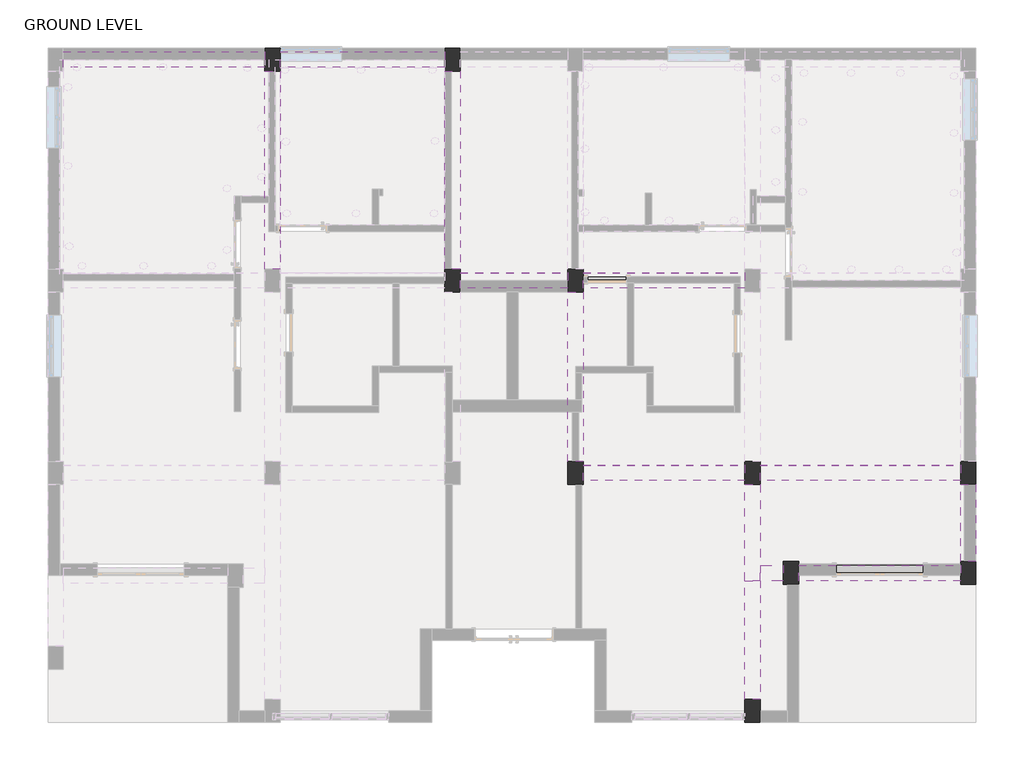
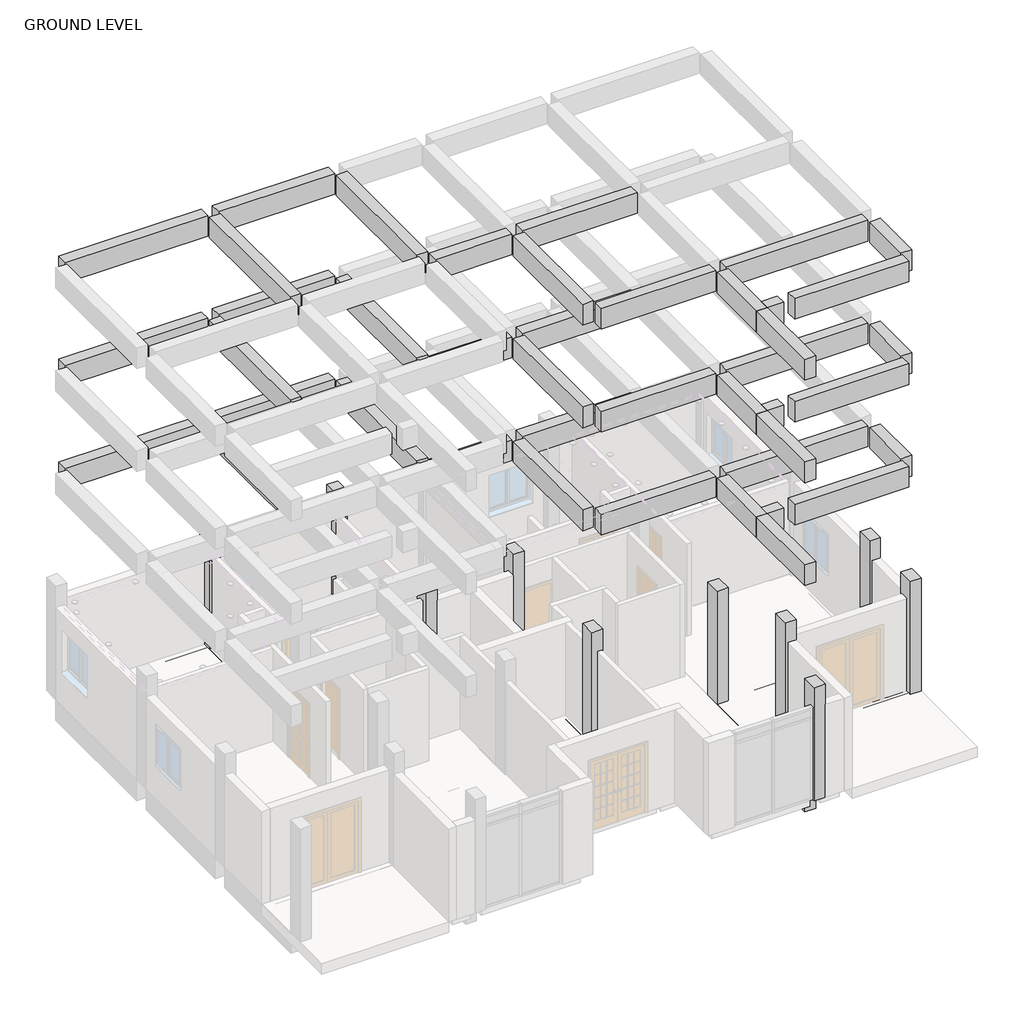
# One storey, part 4 of 5: 57 beams, 10 columns.
"""IFC4 building model written with IfcOpenShell, lengths in millimetres."""

from ifc_helpers import new_model, si_unit, frame, origin, origin_with_axes, place, context, project, spatial, polyline, outline, extrude, faceted_brep, element, save

model = new_model("IFC4")

# Units and contexts
model_context = context("Model", 3, world=origin())
ifc_project = project(units=[si_unit("LENGTHUNIT", "METRE", prefix="MILLI")], contexts=[model_context])

# Site, building, storey
site = spatial("IfcSite", under=ifc_project)
building = spatial("IfcBuilding", under=site)
storey = spatial("IfcBuildingStorey", under=building, Name="GROUND LEVEL", Elevation=0.0)

# Beams
placement = place(None, origin())
element("IfcBeam", 1, ObjectType="Concrete-Rectangular Beam : 12 x 24", at=placement, inside=storey, context=model_context, shape_type="SweptSolid", body=[
    extrude(outline(polyline([(-8839.9786397, -1604.6061634), (-8839.9786397, -1299.8061634), (-4852.9175798, -1299.8061634), (-4852.9175798, -1604.6061634), (-8839.9786397, -1604.6061634)])), frame((0.0, 0.0, -609.6), z_axis=(0.0, 0.0, 1.0), x_axis=(1.0, 0.0, 0.0)), (0.0, 0.0, 1.0), 609.6),
])
element("IfcBeam", 2, ObjectType="Concrete-Rectangular Beam : 12 x 24", at=placement, inside=storey, context=model_context, shape_type="SweptSolid", body=[
    extrude(outline(polyline([(-1296.9175798, -1299.8061634), (-1296.9175798, -1604.6061634), (-4548.1175798, -1604.6061634), (-4548.1175798, -1299.8061634), (-1296.9175798, -1299.8061634)])), frame((0.0, 0.0, -609.6), z_axis=(0.0, 0.0, 1.0), x_axis=(1.0, 0.0, 0.0)), (0.0, 0.0, 1.0), 609.6),
])
element("IfcBeam", 3, ObjectType="Concrete-Rectangular Beam : 12 x 24", at=placement, inside=storey, context=model_context, shape_type="SweptSolid", body=[
    extrude(outline(polyline([(9218.6824202, -11391.8620333), (8913.8824202, -11391.8620333), (8913.8824202, -9867.8620333), (9218.6824202, -9867.8620333), (9218.6824202, -11391.8620333)])), frame((0.0, 0.0, -609.6), z_axis=(0.0, 0.0, 1.0), x_axis=(1.0, 0.0, 0.0)), (0.0, 0.0, 1.0), 609.6),
])
element("IfcBeam", 4, ObjectType="Concrete-Rectangular Beam : 12 x 24", at=placement, inside=storey, context=model_context, shape_type="SweptSolid", body=[
    extrude(outline(polyline([(1446.2824202, -5981.6620333), (1446.2824202, -5676.8620333), (4646.6824202, -5676.8620333), (4646.6824202, -5981.6620333), (1446.2824202, -5981.6620333)])), frame((0.0, 0.0, -609.6), z_axis=(0.0, 0.0, 1.0), x_axis=(1.0, 0.0, 0.0)), (0.0, 0.0, 1.0), 609.6),
])
element("IfcBeam", 5, ObjectType="Concrete-Rectangular Beam : 12 x 24", at=placement, inside=storey, context=model_context, shape_type="SweptSolid", body=[
    extrude(outline(polyline([(-992.1175798, -5981.6620333), (-992.1175798, -5676.8620333), (1141.4824202, -5676.8620333), (1141.4824202, -5981.6620333), (-992.1175798, -5981.6620333)])), frame((0.0, 0.0, -609.6), z_axis=(0.0, 0.0, 1.0), x_axis=(1.0, 0.0, 0.0)), (0.0, 0.0, 1.0), 609.6),
])
element("IfcBeam", 6, ObjectType="Concrete-Rectangular Beam : 12 x 24", at=placement, inside=storey, context=model_context, shape_type="SweptSolid", body=[
    extrude(outline(polyline([(1141.4824202, -9486.8620333), (1141.4824202, -9791.6620333), (-992.1175798, -9791.6620333), (-992.1175798, -9486.8620333), (1141.4824202, -9486.8620333)])), frame((0.0, 0.0, -609.6), z_axis=(0.0, 0.0, 1.0), x_axis=(1.0, 0.0, 0.0)), (0.0, 0.0, 1.0), 609.6),
])
element("IfcBeam", 7, ObjectType="Concrete-Rectangular Beam : 12 x 24", at=placement, inside=storey, context=model_context, shape_type="SweptSolid", body=[
    extrude(outline(polyline([(1446.2824202, -9791.6620333), (1446.2824202, -9486.8620333), (4646.6824202, -9486.8620333), (4646.6824202, -9791.6620333), (1446.2824202, -9791.6620333)])), frame((0.0, 0.0, -609.6), z_axis=(0.0, 0.0, 1.0), x_axis=(1.0, 0.0, 0.0)), (0.0, 0.0, 1.0), 609.6),
])
element("IfcBeam", 8, ObjectType="Concrete-Rectangular Beam : 12 x 24", at=placement, inside=storey, context=model_context, shape_type="Brep", body=[
    faceted_brep([(4951.4824202, -9867.8620333, 0.0), (4646.6824202, -9867.8620333, 0.0), (4646.6824202, -11772.8620333, 0.0), (4951.4824202, -11772.8620333, 0.0), (4951.4824202, -11468.0620333, 0.0), (4646.6824202, -9867.8620333, -609.6), (4646.6824202, -11772.8620333, -609.6), (4951.4824202, -9867.8620333, -609.6), (4951.4824202, -11468.0620333, -609.6), (4951.4824202, -11772.8620333, -609.6)], [[[0, 1, 2, 3, 4]], [[1, 5, 6, 2]], [[5, 7, 8, 9, 6]], [[7, 0, 4, 3, 9, 8]], [[0, 7, 5, 1]], [[3, 2, 6, 9]]]),
])
element("IfcBeam", 9, ObjectType="Concrete-Rectangular Beam : 12 x 24", at=placement, inside=storey, context=model_context, shape_type="SweptSolid", body=[
    extrude(outline(polyline([(5408.6824202, -11468.0620333), (5408.6824202, -11772.8620333), (4951.4824202, -11772.8620333), (4951.4824202, -11468.0620333), (5408.6824202, -11468.0620333)])), frame((0.0, 0.0, -609.6), z_axis=(0.0, 0.0, 1.0), x_axis=(1.0, 0.0, 0.0)), (0.0, 0.0, 1.0), 609.6),
])
element("IfcBeam", 10, ObjectType="Concrete-Rectangular Beam : 12 x 24", at=placement, inside=storey, context=model_context, shape_type="SweptSolid", body=[
    extrude(outline(polyline([(8913.8824202, -11468.0620333), (8913.8824202, -11772.8620333), (5713.4824202, -11772.8620333), (5713.4824202, -11468.0620333), (8913.8824202, -11468.0620333)])), frame((0.0, 0.0, -609.6), z_axis=(0.0, 0.0, 1.0), x_axis=(1.0, 0.0, 0.0)), (0.0, 0.0, 1.0), 609.6),
])
element("IfcBeam", 11, ObjectType="Concrete-Rectangular Beam : 12 x 24", at=placement, inside=storey, context=model_context, shape_type="SweptSolid", body=[
    extrude(outline(polyline([(4951.4824202, -14119.6402089), (4646.6824202, -14119.6402089), (4646.6824202, -11772.8620333), (4951.4824202, -11772.8620333), (4951.4824202, -14119.6402089)])), frame((0.0, 0.0, -609.6), z_axis=(0.0, 0.0, 1.0), x_axis=(1.0, 0.0, 0.0)), (0.0, 0.0, 1.0), 609.6),
])
element("IfcBeam", 12, ObjectType="Concrete-Rectangular Beam : 12 x 24", at=placement, inside=storey, context=model_context, shape_type="SweptSolid", body=[
    extrude(outline(polyline([(-4548.1175798, -5600.6620333), (-4852.9175798, -5600.6620333), (-4852.9175798, -1680.8061634), (-4548.1175798, -1680.8061634), (-4548.1175798, -5600.6620333)])), frame((0.0, 0.0, -609.6), z_axis=(0.0, 0.0, 1.0), x_axis=(1.0, 0.0, 0.0)), (0.0, 0.0, 1.0), 609.6),
])
element("IfcBeam", 13, ObjectType="Concrete-Rectangular Beam : 12 x 24", at=placement, inside=storey, context=model_context, shape_type="SweptSolid", body=[
    extrude(outline(polyline([(-992.1175798, -5600.6620333), (-1296.9175798, -5600.6620333), (-1296.9175798, -1680.8061634), (-992.1175798, -1680.8061634), (-992.1175798, -5600.6620333)])), frame((0.0, 0.0, -609.6), z_axis=(0.0, 0.0, 1.0), x_axis=(1.0, 0.0, 0.0)), (0.0, 0.0, 1.0), 609.6),
])
element("IfcBeam", 14, ObjectType="Concrete-Rectangular Beam : 12 x 24", at=placement, inside=storey, context=model_context, shape_type="SweptSolid", body=[
    extrude(outline(polyline([(1141.4824202, -6057.8620333), (1446.2824202, -6057.8620333), (1446.2824202, -9410.6620333), (1141.4824202, -9410.6620333), (1141.4824202, -6057.8620333)])), frame((0.0, 0.0, -609.6), z_axis=(0.0, 0.0, 1.0), x_axis=(1.0, 0.0, 0.0)), (0.0, 0.0, 1.0), 609.6),
])
element("IfcBeam", 15, ObjectType="Concrete-Rectangular Beam : 12 x 24", at=placement, inside=storey, context=model_context, shape_type="SweptSolid", body=[
    extrude(outline(polyline([(4951.4824202, -9791.6620333), (4951.4824202, -9486.8620333), (8913.8824202, -9486.8620333), (8913.8824202, -9791.6620333), (4951.4824202, -9791.6620333)])), frame((0.0, 0.0, -609.6), z_axis=(0.0, 0.0, 1.0), x_axis=(1.0, 0.0, 0.0)), (0.0, 0.0, 1.0), 609.6),
])
element("IfcBeam", 16, ObjectType="Concrete-Rectangular Beam : 12 x 24", at=placement, inside=storey, context=model_context, shape_type="SweptSolid", body=[
    extrude(outline(polyline([(-8839.9786397, -1604.6061634), (-8839.9786397, -1299.8061634), (-4852.9175798, -1299.8061634), (-4852.9175798, -1604.6061634), (-8839.9786397, -1604.6061634)])), frame((0.0, 0.0, 6096.0), z_axis=(0.0, 0.0, 1.0), x_axis=(1.0, 0.0, 0.0)), (0.0, 0.0, 1.0), 609.6),
])
element("IfcBeam", 17, ObjectType="Concrete-Rectangular Beam : 12 x 24", at=placement, inside=storey, context=model_context, shape_type="SweptSolid", body=[
    extrude(outline(polyline([(-1296.9175798, -1299.8061634), (-1296.9175798, -1604.6061634), (-4548.1175798, -1604.6061634), (-4548.1175798, -1299.8061634), (-1296.9175798, -1299.8061634)])), frame((0.0, 0.0, 6096.0), z_axis=(0.0, 0.0, 1.0), x_axis=(1.0, 0.0, 0.0)), (0.0, 0.0, 1.0), 609.6),
])
element("IfcBeam", 18, ObjectType="Concrete-Rectangular Beam : 12 x 24", at=placement, inside=storey, context=model_context, shape_type="Brep", body=[
    faceted_brep([(8913.8824202, -11391.8620333, 6705.6), (9218.6824202, -11391.8620333, 6705.6), (9218.6824202, -9867.8620333, 6705.6), (8913.8824202, -9867.8620333, 6705.6), (8913.8824202, -11391.8620333, 6096.0), (8913.8824202, -11391.8620333, 6400.8), (8913.8824202, -9867.8620333, 6400.8), (8913.8824202, -9867.8620333, 6096.0), (9218.6824202, -11391.8620333, 6096.0), (9218.6824202, -9867.8620333, 6096.0), (9218.6824202, -11391.8620333, 6400.8), (9218.6824202, -9867.8620333, 6400.8)], [[[0, 1, 2, 3]], [[4, 5, 0, 3, 6, 7]], [[8, 4, 7, 9]], [[1, 10, 8, 9, 11, 2]], [[1, 0, 5, 4, 8, 10]], [[2, 11, 9, 7, 6, 3]]]),
])
element("IfcBeam", 19, ObjectType="Concrete-Rectangular Beam : 12 x 24", at=placement, inside=storey, context=model_context, shape_type="SweptSolid", body=[
    extrude(outline(polyline([(1446.2824202, -5981.6620333), (1446.2824202, -5676.8620333), (4646.6824202, -5676.8620333), (4646.6824202, -5981.6620333), (1446.2824202, -5981.6620333)])), frame((0.0, 0.0, 6096.0), z_axis=(0.0, 0.0, 1.0), x_axis=(1.0, 0.0, 0.0)), (0.0, 0.0, 1.0), 609.6),
])
element("IfcBeam", 20, ObjectType="Concrete-Rectangular Beam : 12 x 24", at=placement, inside=storey, context=model_context, shape_type="SweptSolid", body=[
    extrude(outline(polyline([(-992.1175798, -5981.6620333), (-992.1175798, -5676.8620333), (1141.4824202, -5676.8620333), (1141.4824202, -5981.6620333), (-992.1175798, -5981.6620333)])), frame((0.0, 0.0, 6096.0), z_axis=(0.0, 0.0, 1.0), x_axis=(1.0, 0.0, 0.0)), (0.0, 0.0, 1.0), 609.6),
])
element("IfcBeam", 21, ObjectType="Concrete-Rectangular Beam : 12 x 24", at=placement, inside=storey, context=model_context, shape_type="SweptSolid", body=[
    extrude(outline(polyline([(1446.2824202, -9791.6620333), (1446.2824202, -9486.8620333), (4646.6824202, -9486.8620333), (4646.6824202, -9791.6620333), (1446.2824202, -9791.6620333)])), frame((0.0, 0.0, 6096.0), z_axis=(0.0, 0.0, 1.0), x_axis=(1.0, 0.0, 0.0)), (0.0, 0.0, 1.0), 609.6),
])
element("IfcBeam", 22, ObjectType="Concrete-Rectangular Beam : 12 x 24", at=placement, inside=storey, context=model_context, shape_type="Brep", body=[
    faceted_brep([(4951.4824202, -9867.8620333, 6705.6), (4646.6824202, -9867.8620333, 6705.6), (4646.6824202, -11772.8620333, 6705.6), (4951.4824202, -11772.8620333, 6705.6), (4951.4824202, -11468.0620333, 6705.6), (4646.6824202, -9867.8620333, 6400.8), (4646.6824202, -9867.8620333, 6096.0), (4646.6824202, -11772.8620333, 6096.0), (4951.4824202, -9867.8620333, 6096.0), (4951.4824202, -11468.0620333, 6096.0), (4951.4824202, -11772.8620333, 6096.0), (4951.4824202, -9867.8620333, 6400.8)], [[[0, 1, 2, 3, 4]], [[1, 5, 6, 7, 2]], [[6, 8, 9, 10, 7]], [[8, 11, 0, 4, 3, 10, 9]], [[0, 11, 8, 6, 5, 1]], [[3, 2, 7, 10]]]),
])
element("IfcBeam", 23, ObjectType="Concrete-Rectangular Beam : 12 x 24", at=placement, inside=storey, context=model_context, shape_type="SweptSolid", body=[
    extrude(outline(polyline([(5408.6824202, -11468.0620333), (5408.6824202, -11772.8620333), (4951.4824202, -11772.8620333), (4951.4824202, -11468.0620333), (5408.6824202, -11468.0620333)])), frame((0.0, 0.0, 6096.0), z_axis=(0.0, 0.0, 1.0), x_axis=(1.0, 0.0, 0.0)), (0.0, 0.0, 1.0), 609.6),
])
element("IfcBeam", 24, ObjectType="Concrete-Rectangular Beam : 12 x 24", at=placement, inside=storey, context=model_context, shape_type="SweptSolid", body=[
    extrude(outline(polyline([(8913.8824202, -11468.0620333), (8913.8824202, -11772.8620333), (5713.4824202, -11772.8620333), (5713.4824202, -11468.0620333), (8913.8824202, -11468.0620333)])), frame((0.0, 0.0, 6096.0), z_axis=(0.0, 0.0, 1.0), x_axis=(1.0, 0.0, 0.0)), (0.0, 0.0, 1.0), 609.6),
])
element("IfcBeam", 25, ObjectType="Concrete-Rectangular Beam : 12 x 24", at=placement, inside=storey, context=model_context, shape_type="Brep", body=[
    faceted_brep([(4646.6824202, -14119.6402089, 6705.6), (4951.4824202, -14119.6402089, 6705.6), (4951.4824202, -11772.8620333, 6705.6), (4646.6824202, -11772.8620333, 6705.6), (4951.4824202, -14119.6402089, 6400.8), (4951.4824202, -14119.6402089, 6096.0), (4951.4824202, -11772.8620333, 6096.0), (4646.6824202, -14119.6402089, 6096.0), (4646.6824202, -11772.8620333, 6096.0), (4646.6824202, -14119.6402089, 6400.8)], [[[0, 1, 2, 3]], [[1, 4, 5, 6, 2]], [[5, 7, 8, 6]], [[7, 9, 0, 3, 8]], [[0, 9, 7, 5, 4, 1]], [[3, 2, 6, 8]]]),
])
element("IfcBeam", 26, ObjectType="Concrete-Rectangular Beam : 12 x 24", at=placement, inside=storey, context=model_context, shape_type="Brep", body=[
    faceted_brep([(-4852.9175798, -5600.6620333, 6705.6), (-4548.1175798, -5600.6620333, 6705.6), (-4548.1175798, -1680.8061634, 6705.6), (-4852.9175798, -1680.8061634, 6705.6), (-4852.9175798, -5600.6620333, 6096.0), (-4852.9175798, -5600.6620333, 6400.8), (-4852.9175798, -1680.8061634, 6400.8), (-4852.9175798, -1680.8061634, 6096.0), (-4548.1175798, -5600.6620333, 6096.0), (-4548.1175798, -1680.8061634, 6096.0), (-4548.1175798, -5600.6620333, 6400.8), (-4548.1175798, -1680.8061634, 6400.8)], [[[0, 1, 2, 3]], [[4, 5, 0, 3, 6, 7]], [[8, 4, 7, 9]], [[1, 10, 8, 9, 11, 2]], [[2, 11, 9, 7, 6, 3]], [[1, 0, 5, 4, 8, 10]]]),
])
element("IfcBeam", 27, ObjectType="Concrete-Rectangular Beam : 12 x 24", at=placement, inside=storey, context=model_context, shape_type="Brep", body=[
    faceted_brep([(-1296.9175798, -5600.6620333, 6705.6), (-992.1175798, -5600.6620333, 6705.6), (-992.1175798, -1680.8061634, 6705.6), (-1296.9175798, -1680.8061634, 6705.6), (-1296.9175798, -5600.6620333, 6096.0), (-1296.9175798, -5600.6620333, 6400.8), (-1296.9175798, -1680.8061634, 6400.8), (-1296.9175798, -1680.8061634, 6096.0), (-992.1175798, -5600.6620333, 6096.0), (-992.1175798, -1680.8061634, 6096.0), (-992.1175798, -5600.6620333, 6400.8), (-992.1175798, -1680.8061634, 6400.8)], [[[0, 1, 2, 3]], [[4, 5, 0, 3, 6, 7]], [[8, 4, 7, 9]], [[1, 10, 8, 9, 11, 2]], [[2, 11, 9, 7, 6, 3]], [[1, 0, 5, 4, 8, 10]]]),
])
element("IfcBeam", 28, ObjectType="Concrete-Rectangular Beam : 12 x 24", at=placement, inside=storey, context=model_context, shape_type="Brep", body=[
    faceted_brep([(1446.2824202, -6057.8620333, 6705.6), (1141.4824202, -6057.8620333, 6705.6), (1141.4824202, -9410.6620333, 6705.6), (1446.2824202, -9410.6620333, 6705.6), (1446.2824202, -6057.8620333, 6096.0), (1446.2824202, -6057.8620333, 6400.8), (1446.2824202, -9410.6620333, 6400.8), (1446.2824202, -9410.6620333, 6096.0), (1141.4824202, -6057.8620333, 6096.0), (1141.4824202, -9410.6620333, 6096.0), (1141.4824202, -6057.8620333, 6400.8), (1141.4824202, -9410.6620333, 6400.8)], [[[0, 1, 2, 3]], [[4, 5, 0, 3, 6, 7]], [[8, 4, 7, 9]], [[1, 10, 8, 9, 11, 2]], [[1, 0, 5, 4, 8, 10]], [[2, 11, 9, 7, 6, 3]]]),
])
element("IfcBeam", 29, ObjectType="Concrete-Rectangular Beam : 12 x 24", at=placement, inside=storey, context=model_context, shape_type="SweptSolid", body=[
    extrude(outline(polyline([(4951.4824202, -9791.6620333), (4951.4824202, -9486.8620333), (8913.8824202, -9486.8620333), (8913.8824202, -9791.6620333), (4951.4824202, -9791.6620333)])), frame((0.0, 0.0, 6096.0), z_axis=(0.0, 0.0, 1.0), x_axis=(1.0, 0.0, 0.0)), (0.0, 0.0, 1.0), 609.6),
])
element("IfcBeam", 30, ObjectType="Concrete-Rectangular Beam : 12 x 24", at=placement, inside=storey, context=model_context, shape_type="SweptSolid", body=[
    extrude(outline(polyline([(-8839.9786397, -1604.6061634), (-8839.9786397, -1299.8061634), (-4852.9175798, -1299.8061634), (-4852.9175798, -1604.6061634), (-8839.9786397, -1604.6061634)])), frame((0.0, 0.0, 9144.0), z_axis=(0.0, 0.0, 1.0), x_axis=(1.0, 0.0, 0.0)), (0.0, 0.0, 1.0), 609.6),
])
element("IfcBeam", 31, ObjectType="Concrete-Rectangular Beam : 12 x 24", at=placement, inside=storey, context=model_context, shape_type="SweptSolid", body=[
    extrude(outline(polyline([(-1296.9175798, -1299.8061634), (-1296.9175798, -1604.6061634), (-4548.1175798, -1604.6061634), (-4548.1175798, -1299.8061634), (-1296.9175798, -1299.8061634)])), frame((0.0, 0.0, 9144.0), z_axis=(0.0, 0.0, 1.0), x_axis=(1.0, 0.0, 0.0)), (0.0, 0.0, 1.0), 609.6),
])
element("IfcBeam", 32, ObjectType="Concrete-Rectangular Beam : 12 x 24", at=placement, inside=storey, context=model_context, shape_type="Brep", body=[
    faceted_brep([(8913.8824202, -11391.8620333, 9753.6), (9218.6824202, -11391.8620333, 9753.6), (9218.6824202, -9867.8620333, 9753.6), (8913.8824202, -9867.8620333, 9753.6), (8913.8824202, -11391.8620333, 9144.0), (8913.8824202, -11391.8620333, 9448.8), (8913.8824202, -9867.8620333, 9448.8), (8913.8824202, -9867.8620333, 9144.0), (9218.6824202, -11391.8620333, 9144.0), (9218.6824202, -9867.8620333, 9144.0), (9218.6824202, -11391.8620333, 9448.8), (9218.6824202, -9867.8620333, 9448.8)], [[[0, 1, 2, 3]], [[4, 5, 0, 3, 6, 7]], [[8, 4, 7, 9]], [[1, 10, 8, 9, 11, 2]], [[1, 0, 5, 4, 8, 10]], [[2, 11, 9, 7, 6, 3]]]),
])
element("IfcBeam", 33, ObjectType="Concrete-Rectangular Beam : 12 x 24", at=placement, inside=storey, context=model_context, shape_type="SweptSolid", body=[
    extrude(outline(polyline([(1446.2824202, -5981.6620333), (1446.2824202, -5676.8620333), (4646.6824202, -5676.8620333), (4646.6824202, -5981.6620333), (1446.2824202, -5981.6620333)])), frame((0.0, 0.0, 9144.0), z_axis=(0.0, 0.0, 1.0), x_axis=(1.0, 0.0, 0.0)), (0.0, 0.0, 1.0), 609.6),
])
element("IfcBeam", 34, ObjectType="Concrete-Rectangular Beam : 12 x 24", at=placement, inside=storey, context=model_context, shape_type="SweptSolid", body=[
    extrude(outline(polyline([(-992.1175798, -5981.6620333), (-992.1175798, -5676.8620333), (1141.4824202, -5676.8620333), (1141.4824202, -5981.6620333), (-992.1175798, -5981.6620333)])), frame((0.0, 0.0, 9144.0), z_axis=(0.0, 0.0, 1.0), x_axis=(1.0, 0.0, 0.0)), (0.0, 0.0, 1.0), 609.6),
])
element("IfcBeam", 35, ObjectType="Concrete-Rectangular Beam : 12 x 24", at=placement, inside=storey, context=model_context, shape_type="SweptSolid", body=[
    extrude(outline(polyline([(1446.2824202, -9791.6620333), (1446.2824202, -9486.8620333), (4646.6824202, -9486.8620333), (4646.6824202, -9791.6620333), (1446.2824202, -9791.6620333)])), frame((0.0, 0.0, 9144.0), z_axis=(0.0, 0.0, 1.0), x_axis=(1.0, 0.0, 0.0)), (0.0, 0.0, 1.0), 609.6),
])
element("IfcBeam", 36, ObjectType="Concrete-Rectangular Beam : 12 x 24", at=placement, inside=storey, context=model_context, shape_type="Brep", body=[
    faceted_brep([(4951.4824202, -9867.8620333, 9753.6), (4646.6824202, -9867.8620333, 9753.6), (4646.6824202, -11772.8620333, 9753.6), (4951.4824202, -11772.8620333, 9753.6), (4951.4824202, -11468.0620333, 9753.6), (4646.6824202, -9867.8620333, 9448.8), (4646.6824202, -9867.8620333, 9144.0), (4646.6824202, -11772.8620333, 9144.0), (4951.4824202, -9867.8620333, 9144.0), (4951.4824202, -11468.0620333, 9144.0), (4951.4824202, -11772.8620333, 9144.0), (4951.4824202, -9867.8620333, 9448.8)], [[[0, 1, 2, 3, 4]], [[1, 5, 6, 7, 2]], [[6, 8, 9, 10, 7]], [[8, 11, 0, 4, 3, 10, 9]], [[0, 11, 8, 6, 5, 1]], [[3, 2, 7, 10]]]),
])
element("IfcBeam", 37, ObjectType="Concrete-Rectangular Beam : 12 x 24", at=placement, inside=storey, context=model_context, shape_type="SweptSolid", body=[
    extrude(outline(polyline([(5408.6824202, -11468.0620333), (5408.6824202, -11772.8620333), (4951.4824202, -11772.8620333), (4951.4824202, -11468.0620333), (5408.6824202, -11468.0620333)])), frame((0.0, 0.0, 9144.0), z_axis=(0.0, 0.0, 1.0), x_axis=(1.0, 0.0, 0.0)), (0.0, 0.0, 1.0), 609.6),
])
element("IfcBeam", 38, ObjectType="Concrete-Rectangular Beam : 12 x 24", at=placement, inside=storey, context=model_context, shape_type="SweptSolid", body=[
    extrude(outline(polyline([(8913.8824202, -11468.0620333), (8913.8824202, -11772.8620333), (5713.4824202, -11772.8620333), (5713.4824202, -11468.0620333), (8913.8824202, -11468.0620333)])), frame((0.0, 0.0, 9144.0), z_axis=(0.0, 0.0, 1.0), x_axis=(1.0, 0.0, 0.0)), (0.0, 0.0, 1.0), 609.6),
])
element("IfcBeam", 39, ObjectType="Concrete-Rectangular Beam : 12 x 24", at=placement, inside=storey, context=model_context, shape_type="Brep", body=[
    faceted_brep([(4646.6824202, -14119.6402089, 9753.6), (4951.4824202, -14119.6402089, 9753.6), (4951.4824202, -11772.8620333, 9753.6), (4646.6824202, -11772.8620333, 9753.6), (4951.4824202, -14119.6402089, 9448.8), (4951.4824202, -14119.6402089, 9144.0), (4951.4824202, -11772.8620333, 9144.0), (4646.6824202, -14119.6402089, 9144.0), (4646.6824202, -11772.8620333, 9144.0), (4646.6824202, -14119.6402089, 9448.8)], [[[0, 1, 2, 3]], [[1, 4, 5, 6, 2]], [[5, 7, 8, 6]], [[7, 9, 0, 3, 8]], [[0, 9, 7, 5, 4, 1]], [[3, 2, 6, 8]]]),
])
element("IfcBeam", 40, ObjectType="Concrete-Rectangular Beam : 12 x 24", at=placement, inside=storey, context=model_context, shape_type="Brep", body=[
    faceted_brep([(-4852.9175798, -5600.6620333, 9753.6), (-4548.1175798, -5600.6620333, 9753.6), (-4548.1175798, -1680.8061634, 9753.6), (-4852.9175798, -1680.8061634, 9753.6), (-4852.9175798, -5600.6620333, 9144.0), (-4852.9175798, -5600.6620333, 9448.8), (-4852.9175798, -1680.8061634, 9448.8), (-4852.9175798, -1680.8061634, 9144.0), (-4548.1175798, -5600.6620333, 9144.0), (-4548.1175798, -1680.8061634, 9144.0), (-4548.1175798, -5600.6620333, 9448.8), (-4548.1175798, -1680.8061634, 9448.8)], [[[0, 1, 2, 3]], [[4, 5, 0, 3, 6, 7]], [[8, 4, 7, 9]], [[1, 10, 8, 9, 11, 2]], [[2, 11, 9, 7, 6, 3]], [[1, 0, 5, 4, 8, 10]]]),
])
element("IfcBeam", 41, ObjectType="Concrete-Rectangular Beam : 12 x 24", at=placement, inside=storey, context=model_context, shape_type="Brep", body=[
    faceted_brep([(-1296.9175798, -5600.6620333, 9753.6), (-992.1175798, -5600.6620333, 9753.6), (-992.1175798, -1680.8061634, 9753.6), (-1296.9175798, -1680.8061634, 9753.6), (-1296.9175798, -5600.6620333, 9144.0), (-1296.9175798, -5600.6620333, 9448.8), (-1296.9175798, -1680.8061634, 9448.8), (-1296.9175798, -1680.8061634, 9144.0), (-992.1175798, -5600.6620333, 9144.0), (-992.1175798, -1680.8061634, 9144.0), (-992.1175798, -5600.6620333, 9448.8), (-992.1175798, -1680.8061634, 9448.8)], [[[0, 1, 2, 3]], [[4, 5, 0, 3, 6, 7]], [[8, 4, 7, 9]], [[1, 10, 8, 9, 11, 2]], [[2, 11, 9, 7, 6, 3]], [[1, 0, 5, 4, 8, 10]]]),
])
element("IfcBeam", 42, ObjectType="Concrete-Rectangular Beam : 12 x 24", at=placement, inside=storey, context=model_context, shape_type="Brep", body=[
    faceted_brep([(1446.2824202, -6057.8620333, 9753.6), (1141.4824202, -6057.8620333, 9753.6), (1141.4824202, -9410.6620333, 9753.6), (1446.2824202, -9410.6620333, 9753.6), (1446.2824202, -6057.8620333, 9144.0), (1446.2824202, -6057.8620333, 9448.8), (1446.2824202, -9410.6620333, 9448.8), (1446.2824202, -9410.6620333, 9144.0), (1141.4824202, -6057.8620333, 9144.0), (1141.4824202, -9410.6620333, 9144.0), (1141.4824202, -6057.8620333, 9448.8), (1141.4824202, -9410.6620333, 9448.8)], [[[0, 1, 2, 3]], [[4, 5, 0, 3, 6, 7]], [[8, 4, 7, 9]], [[1, 10, 8, 9, 11, 2]], [[1, 0, 5, 4, 8, 10]], [[2, 11, 9, 7, 6, 3]]]),
])
element("IfcBeam", 43, ObjectType="Concrete-Rectangular Beam : 12 x 24", at=placement, inside=storey, context=model_context, shape_type="SweptSolid", body=[
    extrude(outline(polyline([(4951.4824202, -9791.6620333), (4951.4824202, -9486.8620333), (8913.8824202, -9486.8620333), (8913.8824202, -9791.6620333), (4951.4824202, -9791.6620333)])), frame((0.0, 0.0, 9144.0), z_axis=(0.0, 0.0, 1.0), x_axis=(1.0, 0.0, 0.0)), (0.0, 0.0, 1.0), 609.6),
])
element("IfcBeam", 44, ObjectType="Concrete-Rectangular Beam : 12 x 24", at=placement, inside=storey, context=model_context, shape_type="SweptSolid", body=[
    extrude(outline(polyline([(-8839.9786397, -1604.6061634), (-8839.9786397, -1299.8061634), (-4852.9175798, -1299.8061634), (-4852.9175798, -1604.6061634), (-8839.9786397, -1604.6061634)])), frame((0.0, 0.0, 12192.0), z_axis=(0.0, 0.0, 1.0), x_axis=(1.0, 0.0, 0.0)), (0.0, 0.0, 1.0), 609.6),
])
element("IfcBeam", 45, ObjectType="Concrete-Rectangular Beam : 12 x 24", at=placement, inside=storey, context=model_context, shape_type="SweptSolid", body=[
    extrude(outline(polyline([(-1296.9175798, -1299.8061634), (-1296.9175798, -1604.6061634), (-4548.1175798, -1604.6061634), (-4548.1175798, -1299.8061634), (-1296.9175798, -1299.8061634)])), frame((0.0, 0.0, 12192.0), z_axis=(0.0, 0.0, 1.0), x_axis=(1.0, 0.0, 0.0)), (0.0, 0.0, 1.0), 609.6),
])
element("IfcBeam", 46, ObjectType="Concrete-Rectangular Beam : 12 x 24", at=placement, inside=storey, context=model_context, shape_type="SweptSolid", body=[
    extrude(outline(polyline([(9218.6824202, -11391.8620333), (8913.8824202, -11391.8620333), (8913.8824202, -9867.8620333), (9218.6824202, -9867.8620333), (9218.6824202, -11391.8620333)])), frame((0.0, 0.0, 12192.0), z_axis=(0.0, 0.0, 1.0), x_axis=(1.0, 0.0, 0.0)), (0.0, 0.0, 1.0), 609.6),
])
element("IfcBeam", 47, ObjectType="Concrete-Rectangular Beam : 12 x 24", at=placement, inside=storey, context=model_context, shape_type="SweptSolid", body=[
    extrude(outline(polyline([(1446.2824202, -5981.6620333), (1446.2824202, -5676.8620333), (4646.6824202, -5676.8620333), (4646.6824202, -5981.6620333), (1446.2824202, -5981.6620333)])), frame((0.0, 0.0, 12192.0), z_axis=(0.0, 0.0, 1.0), x_axis=(1.0, 0.0, 0.0)), (0.0, 0.0, 1.0), 609.6),
])
element("IfcBeam", 48, ObjectType="Concrete-Rectangular Beam : 12 x 24", at=placement, inside=storey, context=model_context, shape_type="SweptSolid", body=[
    extrude(outline(polyline([(-992.1175798, -5981.6620333), (-992.1175798, -5676.8620333), (1141.4824202, -5676.8620333), (1141.4824202, -5981.6620333), (-992.1175798, -5981.6620333)])), frame((0.0, 0.0, 12192.0), z_axis=(0.0, 0.0, 1.0), x_axis=(1.0, 0.0, 0.0)), (0.0, 0.0, 1.0), 609.6),
])
element("IfcBeam", 49, ObjectType="Concrete-Rectangular Beam : 12 x 24", at=placement, inside=storey, context=model_context, shape_type="SweptSolid", body=[
    extrude(outline(polyline([(1446.2824202, -9791.6620333), (1446.2824202, -9486.8620333), (4646.6824202, -9486.8620333), (4646.6824202, -9791.6620333), (1446.2824202, -9791.6620333)])), frame((0.0, 0.0, 12192.0), z_axis=(0.0, 0.0, 1.0), x_axis=(1.0, 0.0, 0.0)), (0.0, 0.0, 1.0), 609.6),
])
element("IfcBeam", 50, ObjectType="Concrete-Rectangular Beam : 12 x 24", at=placement, inside=storey, context=model_context, shape_type="Brep", body=[
    faceted_brep([(4951.4824202, -9867.8620333, 12801.6), (4646.6824202, -9867.8620333, 12801.6), (4646.6824202, -11772.8620333, 12801.6), (4951.4824202, -11772.8620333, 12801.6), (4951.4824202, -11468.0620333, 12801.6), (4646.6824202, -9867.8620333, 12192.0), (4646.6824202, -11772.8620333, 12192.0), (4951.4824202, -9867.8620333, 12192.0), (4951.4824202, -11468.0620333, 12192.0), (4951.4824202, -11772.8620333, 12192.0)], [[[0, 1, 2, 3, 4]], [[1, 5, 6, 2]], [[5, 7, 8, 9, 6]], [[7, 0, 4, 3, 9, 8]], [[3, 2, 6, 9]], [[0, 7, 5, 1]]]),
])
element("IfcBeam", 51, ObjectType="Concrete-Rectangular Beam : 12 x 24", at=placement, inside=storey, context=model_context, shape_type="SweptSolid", body=[
    extrude(outline(polyline([(5408.6824202, -11468.0620333), (5408.6824202, -11772.8620333), (4951.4824202, -11772.8620333), (4951.4824202, -11468.0620333), (5408.6824202, -11468.0620333)])), frame((0.0, 0.0, 12192.0), z_axis=(0.0, 0.0, 1.0), x_axis=(1.0, 0.0, 0.0)), (0.0, 0.0, 1.0), 609.6),
])
element("IfcBeam", 52, ObjectType="Concrete-Rectangular Beam : 12 x 24", at=placement, inside=storey, context=model_context, shape_type="SweptSolid", body=[
    extrude(outline(polyline([(8913.8824202, -11468.0620333), (8913.8824202, -11772.8620333), (5713.4824202, -11772.8620333), (5713.4824202, -11468.0620333), (8913.8824202, -11468.0620333)])), frame((0.0, 0.0, 12192.0), z_axis=(0.0, 0.0, 1.0), x_axis=(1.0, 0.0, 0.0)), (0.0, 0.0, 1.0), 609.6),
])
element("IfcBeam", 53, ObjectType="Concrete-Rectangular Beam : 12 x 24", at=placement, inside=storey, context=model_context, shape_type="SweptSolid", body=[
    extrude(outline(polyline([(4951.4824202, -14119.6402089), (4646.6824202, -14119.6402089), (4646.6824202, -11772.8620333), (4951.4824202, -11772.8620333), (4951.4824202, -14119.6402089)])), frame((0.0, 0.0, 12192.0), z_axis=(0.0, 0.0, 1.0), x_axis=(1.0, 0.0, 0.0)), (0.0, 0.0, 1.0), 609.6),
])
element("IfcBeam", 54, ObjectType="Concrete-Rectangular Beam : 12 x 24", at=placement, inside=storey, context=model_context, shape_type="SweptSolid", body=[
    extrude(outline(polyline([(-4548.1175798, -5600.6620333), (-4852.9175798, -5600.6620333), (-4852.9175798, -1680.8061634), (-4548.1175798, -1680.8061634), (-4548.1175798, -5600.6620333)])), frame((0.0, 0.0, 12192.0), z_axis=(0.0, 0.0, 1.0), x_axis=(1.0, 0.0, 0.0)), (0.0, 0.0, 1.0), 609.6),
])
element("IfcBeam", 55, ObjectType="Concrete-Rectangular Beam : 12 x 24", at=placement, inside=storey, context=model_context, shape_type="SweptSolid", body=[
    extrude(outline(polyline([(-992.1175798, -5600.6620333), (-1296.9175798, -5600.6620333), (-1296.9175798, -1680.8061634), (-992.1175798, -1680.8061634), (-992.1175798, -5600.6620333)])), frame((0.0, 0.0, 12192.0), z_axis=(0.0, 0.0, 1.0), x_axis=(1.0, 0.0, 0.0)), (0.0, 0.0, 1.0), 609.6),
])
element("IfcBeam", 56, ObjectType="Concrete-Rectangular Beam : 12 x 24", at=placement, inside=storey, context=model_context, shape_type="SweptSolid", body=[
    extrude(outline(polyline([(1141.4824202, -6057.8620333), (1446.2824202, -6057.8620333), (1446.2824202, -9410.6620333), (1141.4824202, -9410.6620333), (1141.4824202, -6057.8620333)])), frame((0.0, 0.0, 12192.0), z_axis=(0.0, 0.0, 1.0), x_axis=(1.0, 0.0, 0.0)), (0.0, 0.0, 1.0), 609.6),
])
element("IfcBeam", 57, ObjectType="Concrete-Rectangular Beam : 12 x 24", at=placement, inside=storey, context=model_context, shape_type="SweptSolid", body=[
    extrude(outline(polyline([(4951.4824202, -9791.6620333), (4951.4824202, -9486.8620333), (8913.8824202, -9486.8620333), (8913.8824202, -9791.6620333), (4951.4824202, -9791.6620333)])), frame((0.0, 0.0, 12192.0), z_axis=(0.0, 0.0, 1.0), x_axis=(1.0, 0.0, 0.0)), (0.0, 0.0, 1.0), 609.6),
])

# Columns
element("IfcColumn", 58, ObjectType="Concrete-Rectangular-Column : 1'6\" X 1' COLUMN", at=placement, inside=storey, context=model_context, shape_type="SweptSolid", body=[
    extrude(outline(polyline([(-4548.1175798, -1223.6061634), (-4548.1175798, -1680.8061634), (-4852.9175798, -1680.8061634), (-4852.9175798, -1223.6061634), (-4548.1175798, -1223.6061634)])), origin_with_axes(), (0.0, 0.0, 1.0), 3352.8),
])
element("IfcColumn", 59, ObjectType="Concrete-Rectangular-Column : 1'6\" X 1' COLUMN", at=placement, inside=storey, context=model_context, shape_type="SweptSolid", body=[
    extrude(outline(polyline([(-992.1175798, -1223.6061634), (-992.1175798, -1680.8061634), (-1296.9175798, -1680.8061634), (-1296.9175798, -1223.6061634), (-992.1175798, -1223.6061634)])), origin_with_axes(), (0.0, 0.0, 1.0), 3352.8),
])
element("IfcColumn", 60, ObjectType="Concrete-Rectangular-Column : 1'6\" X 1' COLUMN", at=placement, inside=storey, context=model_context, shape_type="SweptSolid", body=[
    extrude(outline(polyline([(1446.2824202, -5600.6620333), (1446.2824202, -6057.8620333), (1141.4824202, -6057.8620333), (1141.4824202, -5600.6620333), (1446.2824202, -5600.6620333)])), origin_with_axes(), (0.0, 0.0, 1.0), 3352.8),
])
element("IfcColumn", 61, ObjectType="Concrete-Rectangular-Column : 1'6\" X 1' COLUMN", at=placement, inside=storey, context=model_context, shape_type="SweptSolid", body=[
    extrude(outline(polyline([(-992.1175798, -5600.6620333), (-992.1175798, -6057.8620333), (-1296.9175798, -6057.8620333), (-1296.9175798, -5600.6620333), (-992.1175798, -5600.6620333)])), origin_with_axes(), (0.0, 0.0, 1.0), 3352.8),
])
element("IfcColumn", 62, ObjectType="Concrete-Rectangular-Column : 1'6\" X 1' COLUMN", at=placement, inside=storey, context=model_context, shape_type="SweptSolid", body=[
    extrude(outline(polyline([(9218.6824202, -11391.8620333), (9218.6824202, -11849.0620333), (8913.8824202, -11849.0620333), (8913.8824202, -11391.8620333), (9218.6824202, -11391.8620333)])), origin_with_axes(), (0.0, 0.0, 1.0), 3352.8),
])
element("IfcColumn", 63, ObjectType="Concrete-Rectangular-Column : 1'6\" X 1' COLUMN", at=placement, inside=storey, context=model_context, shape_type="SweptSolid", body=[
    extrude(outline(polyline([(9218.6824202, -9410.6620333), (9218.6824202, -9867.8620333), (8913.8824202, -9867.8620333), (8913.8824202, -9410.6620333), (9218.6824202, -9410.6620333)])), origin_with_axes(), (0.0, 0.0, 1.0), 3352.8),
])
element("IfcColumn", 64, ObjectType="Concrete-Rectangular-Column : 1'6\" X 1' COLUMN", at=placement, inside=storey, context=model_context, shape_type="SweptSolid", body=[
    extrude(outline(polyline([(4951.4824202, -9410.6620333), (4951.4824202, -9867.8620333), (4646.6824202, -9867.8620333), (4646.6824202, -9410.6620333), (4951.4824202, -9410.6620333)])), origin_with_axes(), (0.0, 0.0, 1.0), 3352.8),
])
element("IfcColumn", 65, ObjectType="Concrete-Rectangular-Column : 1'6\" X 1' COLUMN", at=placement, inside=storey, context=model_context, shape_type="SweptSolid", body=[
    extrude(outline(polyline([(1446.2824202, -9410.6620333), (1446.2824202, -9867.8620333), (1141.4824202, -9867.8620333), (1141.4824202, -9410.6620333), (1446.2824202, -9410.6620333)])), origin_with_axes(), (0.0, 0.0, 1.0), 3352.8),
])
element("IfcColumn", 66, ObjectType="Concrete-Rectangular-Column : 1'6\" X 1' COLUMN", at=placement, inside=storey, context=model_context, shape_type="SweptSolid", body=[
    extrude(outline(polyline([(5713.4824202, -11391.8620333), (5713.4824202, -11849.0620333), (5408.6824202, -11849.0620333), (5408.6824202, -11391.8620333), (5713.4824202, -11391.8620333)])), origin_with_axes(), (0.0, 0.0, 1.0), 3352.8),
])
element("IfcColumn", 67, ObjectType="Concrete-Rectangular-Column : 1'6\" X 1' COLUMN", at=placement, inside=storey, context=model_context, shape_type="SweptSolid", body=[
    extrude(outline(polyline([(4951.4824202, -14119.6402089), (4951.4824202, -14576.8402089), (4646.6824202, -14576.8402089), (4646.6824202, -14119.6402089), (4951.4824202, -14119.6402089)])), origin_with_axes(), (0.0, 0.0, 1.0), 3352.8),
])

save(model, "model.ifc")

# Revit data of these elements
# Type "Concrete-Rectangular Beam : 12 x 24"
#   Assembly Code = "B10"
#   Length [instance default] = 5' - 0"
#   b = 1' - 0"
#   h = 2' - 0"
#   Structural Material [instance default] = Concrete, Cast-in-Place gray
# Type "Concrete-Rectangular-Column : 1'6\" X 1' COLUMN"
#   Assembly Code = "B10"
#   b = 1' - 0"
#   h = 1' - 6"
#   Structural Material [instance default] = Concrete, Cast-in-Place gray
# Elements 1, 2, 4, 5, 6, 7, 8, 9, 10, 11, 12, 13, 14, 15, 16, 17, 19, 20, 21, 22, 23, 24, 25, 26, 27, 28, 29, 30, 31, 33, 34, 35, 36, 37, 38, 39, 40, 41, 42, 43, 44, 45, 47, 48, 49, 50, 51, 52, 53, 54, 55, 56, 57 (IfcBeam, "Concrete-Rectangular Beam : 12 x 24")
#   Structural Material = WARM BEIGE COLOUR
#   Phase Created = New Construction
#   Materials on its faces: "WARM BEIGE COLOUR"
# Elements 3, 18, 32, 46 (IfcBeam, "Concrete-Rectangular Beam : 12 x 24")
#   Length = 5' - 0"
#   Structural Material = WARM BEIGE COLOUR
#   Phase Created = New Construction
#   Materials on its faces: "WARM BEIGE COLOUR"
# Elements 58, 59, 60, 61, 62, 63, 64, 65, 66, 67 (IfcColumn, "Concrete-Rectangular-Column : 1'6\" X 1' COLUMN")
#   Structural Material = WARM BEIGE COLOUR
#   Phase Created = New Construction
#   Materials on its faces: "WARM BEIGE COLOUR"
# Materials
#   "Concrete, Cast-in-Place gray": class "Concrete", colour RGB 192 192 192, transparency 0, Description = "Cast-in-place concrete", Cost = 0
#   "WARM BEIGE COLOUR": class "Generic", colour RGB 120 120 120, transparency 0, Cost = 0
